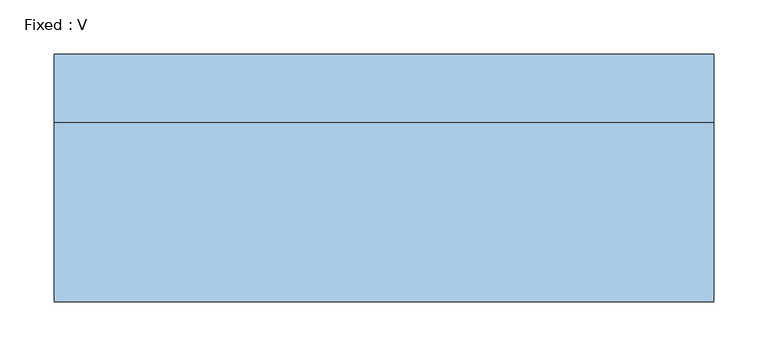
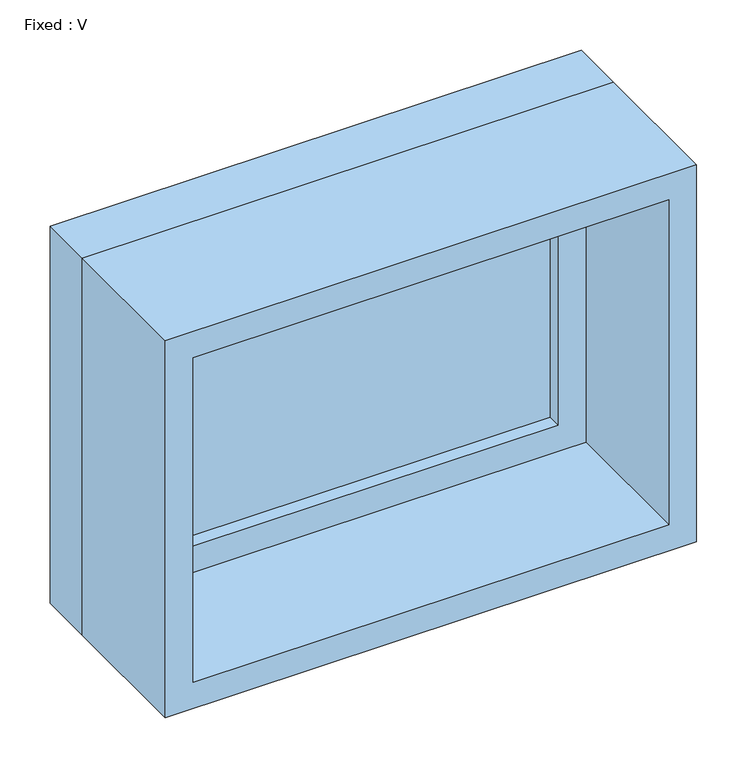
"""IFC4 building model written with IfcOpenShell, lengths in millimetres: window geometry, Fixed : V."""

from ifc_helpers import new_model, si_unit, frame, origin, place, context, project, spatial, polyline, outline, extrude, source, transform, mapped, element, save


def fixed_v_1ea75518(model_context):
    return source(origin(), model_context, "Body", "SweptSolid", [
        extrude(outline(polyline([(203.2, 66.675), (-279.4, 66.675), (-279.4, 79.375), (203.2, 79.375), (203.2, 66.675)])), frame((0.0, 0.0, 977.9), z_axis=(0.0, 0.0, 1.0), x_axis=(1.0, 0.0, 0.0)), (0.0, 0.0, 1.0), 330.2),
        extrude(outline(polyline([(1352.55, -323.85), (933.45, -323.85), (933.45, 247.65), (1352.55, 247.65), (1352.55, -323.85)]), holes=[polyline([(1308.1, -279.4), (1308.1, 203.2), (977.9, 203.2), (977.9, -279.4), (1308.1, -279.4)])]), frame((0.0, 50.8, 0.0), z_axis=(0.0, 1.0, 0.0), x_axis=(0.0, 0.0, 1.0)), (0.0, 0.0, 1.0), 44.45),
        extrude(outline(polyline([(1371.6, -342.9), (914.4, -342.9), (914.4, 266.7), (1371.6, 266.7), (1371.6, -342.9)]), holes=[polyline([(1339.85, -311.15), (1339.85, 234.95), (946.15, 234.95), (946.15, -311.15), (1339.85, -311.15)])]), frame((0.0, -114.3, 0.0), z_axis=(0.0, 1.0, 0.0), x_axis=(0.0, 0.0, 1.0)), (0.0, 0.0, 1.0), 165.1),
        extrude(outline(polyline([(1371.6, 266.7), (1371.6, -342.9), (914.4, -342.9), (914.4, 266.7), (1371.6, 266.7)]), holes=[polyline([(1352.55, 247.65), (933.45, 247.65), (933.45, -323.85), (1352.55, -323.85), (1352.55, 247.65)])]), frame((0.0, 50.8, 0.0), z_axis=(0.0, 1.0, 0.0), x_axis=(0.0, 0.0, 1.0)), (0.0, 0.0, 1.0), 63.5),
    ])


if __name__ == "__main__":
    model = new_model("IFC4")
    model_context = context("Model", 3, world=origin())
    ifc_project = project(units=[si_unit("LENGTHUNIT", "METRE", prefix="MILLI")], contexts=[model_context])
    site = spatial("IfcSite", under=ifc_project)
    building = spatial("IfcBuilding", under=site)
    placement = place(None, origin())
    fixed_v_shape = fixed_v_1ea75518(model_context)
    element("IfcWindow", 1, ObjectType="Fixed : V", at=placement, inside=building, context=model_context, shape_type="MappedRepresentation", body=[
        mapped(fixed_v_shape, transform((0.0, 0.0, 0.0), x_axis=(1.0, 0.0, 0.0), y_axis=(0.0, 1.0, 0.0), z_axis=(0.0, 0.0, 1.0))),
    ])
    save(model, "model.ifc")

# Revit data of these elements
# Type "Fixed : V"
#   Type Mark = "20"
#   Construction Type Id = "GSP4R"
#   Assembly Code = "B2020100"
#   Analytic Construction = "1/8 in Pilkington single glazing"
#   Visual Light Transmittance = 0.9
#   Solar Heat Gain Coefficient = 0.78
#   Heat Transfer Coefficient (U) = 0.6496 BTU/(h·ft²·°F)
#   Height = 1' - 6"
#   Default Sill Height = 3' - 0"
#   Width = 2' - 0"
#   Window Inset = 0' - 0 3/4"
#   Define Thermal Properties by = 1
#   Glass Pane Material = Glass
#   Sash Material = Sash
#   Wall Closure = (empty or 0)
# Element 1 (IfcWindow, "Fixed : V")
#   Materials on its faces: "Sash", "Glass"
# Materials
#   "Glass": class "Glass", colour RGB 0 128 192, transparency 0.75, Description = "Soda Lime Glass", Cost = 0
#   "Sash": class "Wood", colour RGB 224 178 126, transparency 0, Cost = 0
